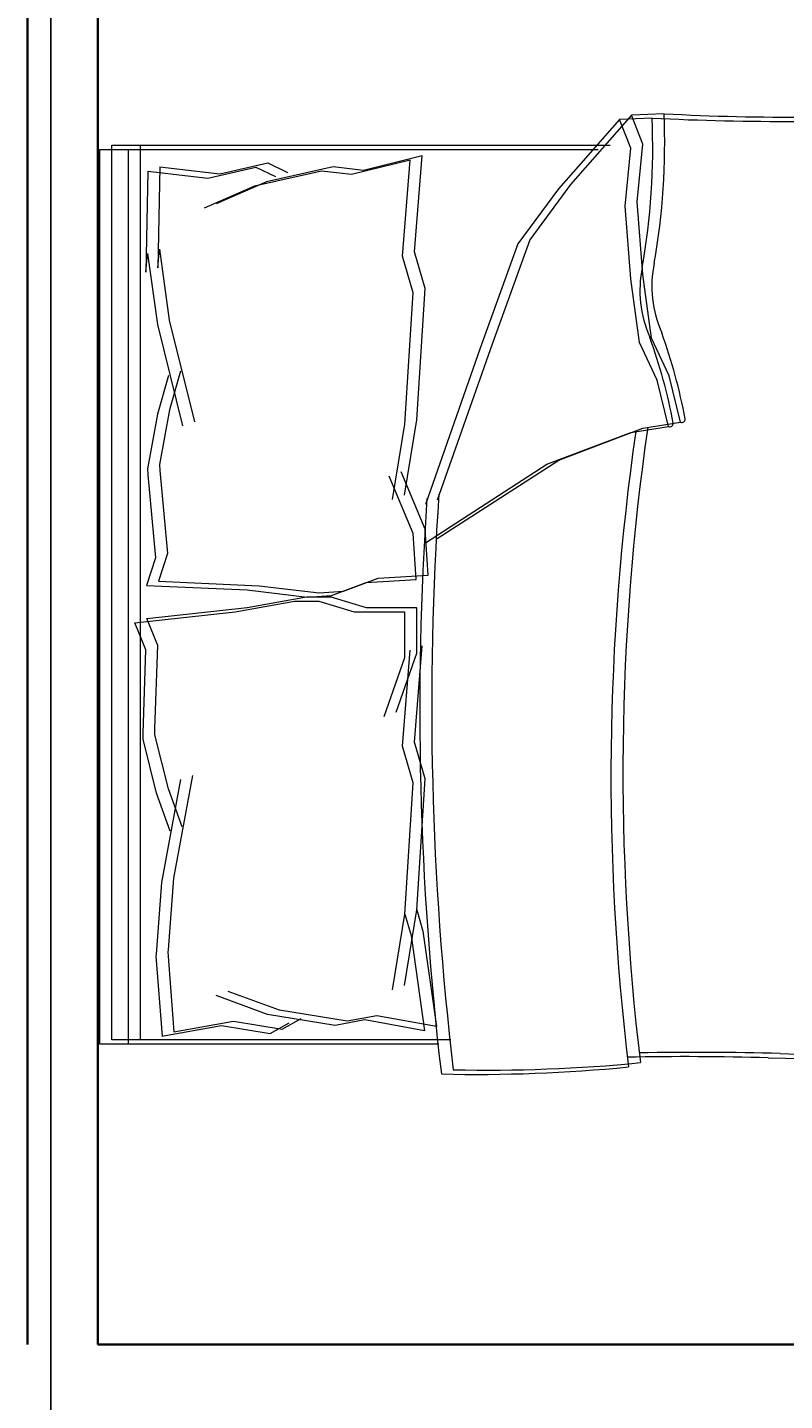
# Model space of a CAD drawing. Units: inches. Extents: x 1088 to 1703, y 668 to 1875.
# Tile 24 of 45: x 1436 to 1484, y 1416 to 1504. Entities that reach past the tile are written whole.
import ezdxf

# ---------------------------------------------------------------- set-up
doc = ezdxf.new("R2010")
doc.units = ezdxf.units.IN
for name, color, linetype, lineweight in [('A-ANNO-DIMS', 2, 'Continuous', 18), ('A-FURN', 8, 'Continuous', 13), ('A-WALL', 7, 'Continuous', 35)]:
    doc.layers.add(name, color=color, linetype=linetype, lineweight=lineweight)
doc.styles.get("Standard").update_dxf_attribs({"font": 'arial.ttf'})
doc.dimstyles.get("Standard").update_dxf_attribs({"dimtxt": 0.18, "dimasz": 0.18, "dimexe": 0.18, "dimexo": 0.0625, "dimgap": 0.09, "dimtad": 0, "dimtih": 1, "dimtoh": 1, "dimdec": 4, "dimzin": 0, "dimdsep": 46, "dimtxsty": 'Standard', "dimcen": 0.09, "dimadec": 0, "dimazin": 0, "dimtfac": 1, "dimtdec": 4, "dimtofl": 0, "dimtmove": 0, "dimatfit": 3, "dimfxl": 1, "dimtolj": 1, "dimtzin": 0, "dimarcsym": 0})

# ---------------------------------------------------------------- blocks, each defined once
blk = doc.blocks.new('BED-DOUBLE')
for p, q in [((33.263, 63.381), (29.367, 58.939)), ((34.03, 63.655), (30.133, 59.213)), ((35.355, 63.476), (33.263, 63.381, 4.641)), ((34.006, 61.538), (33.263, 63.381)), ((36.121, 63.75), (34.03, 63.655, 4.641)), ((34.772, 61.812), (34.03, 63.655)), ((0.766, 61.734), (32.668, 61.734)), ((0.766, 4.44), (0.766, 61.734)), ((2.605, 4.44), (2.605, 61.734)), ((34.401, 58.099), (34.772, 61.812)), ((0, 61.46), (31.901, 61.46)), ((0, 4.167), (0, 61.46)), ((1.838, 4.167), (1.838, 61.46)), ((19.868, 60.78), (16.105, 59.851)), ((20.635, 61.054), (16.872, 60.124)), ((19.384, 54.628), (19.868, 60.78)), ((20.151, 54.902), (20.635, 61.054)), ((33.634, 57.825), (34.006, 61.538)), ((3.065, 60.077), (2.949, 53.601)), ((3.065, 60.077), (6.915, 59.624)), ((3.832, 60.351), (3.716, 53.875)), ((3.832, 60.351), (7.681, 59.897)), ((6.915, 59.624), (9.996, 60.337)), ((7.681, 59.897), (10.763, 60.611)), ((14.181, 60.078), (9.899, 59.115)), ((9.996, 60.337), (11.251, 59.721)), ((14.947, 60.351), (10.665, 59.389)), ((10.763, 60.611), (12.017, 59.995)), ((16.105, 59.851), (14.181, 60.078)), ((16.872, 60.124), (14.947, 60.351)), ((9.899, 59.115), (6.688, 57.699)), ((10.665, 59.389), (7.454, 57.973)), ((29.367, 58.939), (26.769, 55.411)), ((30.133, 59.213), (27.535, 55.685)), ((34.772, 53.457), (34.401, 58.099)), ((34.006, 53.183), (33.634, 57.825)), ((26.769, 55.411), (24.357, 48.727)), ((27.535, 55.685), (25.123, 49.001)), ((2.949, 53.601), (3.048, 54.803)), ((3.048, 54.803), (3.68, 50.25)), ((3.716, 53.875), (3.814, 55.077)), ((3.814, 55.077), (4.446, 50.523)), ((20.052, 52.278), (19.384, 54.628)), ((20.819, 52.552), (20.151, 54.902)), ((34.562, 49.098), (34.006, 53.183)), ((35.329, 49.372), (34.772, 53.457)), ((19.536, 43.874), (20.052, 52.278)), ((20.302, 44.148), (20.819, 52.552)), ((3.68, 50.25), (5.301, 43.753)), ((4.446, 50.523), (6.068, 44.027)), ((36.442, 46.958), (35.329, 49.372)), ((24.357, 48.727), (20.84, 38.731)), ((25.123, 49.001), (21.606, 39.005)), ((35.676, 46.685), (34.562, 49.098)), ((4.404, 46.996), (3.69, 44.52)), ((5.171, 47.27), (4.457, 44.794)), ((36.418, 43.714), (35.676, 46.685)), ((37.184, 43.988), (36.442, 46.958)), ((3.69, 44.52), (3.042, 41.007)), ((4.457, 44.794), (3.808, 41.281)), ((19.503, 39.314), (20.302, 44.148)), ((34.772, 43.616), (37.184, 43.988)), ((18.736, 39.04), (19.536, 43.874)), ((28.624, 41.3), (34.006, 43.342)), ((29.391, 41.574), (34.772, 43.616)), ((34.006, 43.342), (36.418, 43.714)), ((21.606, 36.551), (29.391, 41.574)), ((3.042, 41.007), (3.066, 40.622)), ((3.066, 40.622), (3.571, 35.314)), ((3.808, 41.281), (3.832, 40.896)), ((3.832, 40.896), (4.338, 35.587)), ((20.068, 36.866), (18.528, 40.547)), ((20.835, 37.139), (19.294, 40.82)), ((20.84, 36.277), (28.624, 41.3)), ((21.018, 34.199), (20.835, 37.139)), ((20.252, 33.925), (20.068, 36.866)), ((3.571, 35.314), (2.987, 33.541)), ((4.338, 35.587), (3.754, 33.814)), ((2.987, 33.541), (9.432, 33.249)), ((3.754, 33.814), (10.198, 33.523)), ((10.198, 33.523), (14.047, 33.069)), ((14.838, 32.892), (17.044, 33.725)), ((15.604, 33.166), (17.81, 33.998)), ((17.044, 33.725), (20.252, 33.925)), ((17.81, 33.998), (21.018, 34.199)), ((9.422, 32.117), (13.236, 32.81)), ((9.432, 33.249), (13.281, 32.795)), ((13.236, 32.81), (14.796, 32.81)), ((13.281, 32.795), (14.838, 32.892)), ((14.047, 33.069), (15.604, 33.166)), ((14.796, 32.81), (17.049, 32.117)), ((2.242, 31.15), (8.656, 31.843)), ((3.008, 31.424), (9.422, 32.117)), ((8.656, 31.843), (12.469, 32.536)), ((12.469, 32.536), (14.029, 32.536)), ((14.029, 32.536), (16.283, 31.843)), ((16.283, 31.843), (19.497, 31.843)), ((17.049, 32.117), (20.264, 32.117)), ((19.497, 31.843), (19.497, 28.897)), ((20.264, 32.117), (20.264, 29.171)), ((2.935, 29.417), (2.242, 31.15)), ((3.702, 29.691), (3.008, 31.424)), ((2.762, 24.087), (2.935, 29.417)), ((3.528, 24.361), (3.702, 29.691)), ((20.264, 29.171), (18.956, 25.401)), ((19.384, 23.239), (19.868, 29.391)), ((20.151, 23.513), (20.635, 29.665)), ((19.497, 28.897), (18.189, 25.127)), ((2.762, 23.701), (2.762, 24.087)), ((3.528, 23.975), (3.528, 24.361)), ((4.395, 20.509), (3.528, 23.975)), ((3.629, 20.235), (2.762, 23.701)), ((20.052, 20.889), (19.384, 23.239)), ((20.819, 21.163), (20.151, 23.513)), ((4.742, 14.79), (5.955, 21.376)), ((20.302, 12.759), (20.819, 21.163)), ((4.495, 17.809), (3.629, 20.235)), ((3.975, 14.516), (5.189, 21.102)), ((5.262, 18.083), (4.395, 20.509)), ((19.536, 12.485), (20.052, 20.889)), ((3.629, 9.933), (3.975, 14.516)), ((4.395, 10.206), (4.742, 14.79)), ((18.736, 7.651), (19.536, 12.485)), ((19.503, 7.925), (20.302, 12.759)), ((19.536, 12.485), (19.923, 11.126)), ((20.302, 12.759), (20.689, 11.4)), ((19.923, 11.126), (20.789, 5.016)), ((20.689, 11.4), (21.556, 5.29)), ((3.607, 9.806), (3.629, 9.933)), ((4.002, 4.674), (3.607, 9.806)), ((4.373, 10.08), (4.395, 10.206)), ((4.768, 4.948), (4.373, 10.08)), ((10.736, 6.056), (7.442, 7.269)), ((11.502, 6.33), (8.209, 7.543)), ((15.836, 5.637), (11.502, 6.33)), ((3.975, 4.67), (7.789, 5.363)), ((4.742, 4.943), (8.555, 5.637)), ((7.789, 5.363), (10.909, 4.843)), ((8.555, 5.637), (11.675, 5.117)), ((15.069, 5.363), (10.736, 6.056)), ((10.909, 4.843), (12.122, 5.536)), ((11.675, 5.117), (12.889, 5.81)), ((16.976, 5.709), (15.069, 5.363)), ((17.742, 5.983), (15.836, 5.637)), ((20.789, 5.016), (16.976, 5.709)), ((21.556, 5.29), (17.742, 5.983)), ((22.478, 4.44), (0.766, 4.44)), ((21.712, 4.167), (0, 4.167))]:
    blk.add_line(p, q)
for centre, radius, start, end in [((-7.98, 61.534), 43.378, 349.87628, 2.56571), ((43.537, 218.511), 155.251, 266.97912, 273.83645), ((-7.213, 61.808), 43.378, 349.87628, 2.56571), ((44.303, 218.785), 155.251, 266.97912, 273.83645), ((42.039, 52.443), 7.462, 168.6608, 203.73842), ((42.806, 52.716), 7.462, 168.6608, 203.73842), ((1.777, 37.349), 35.551, 10.66171, 19.88058), ((2.543, 37.623), 35.551, 10.66171, 19.88058), ((37.259, 44.196), 0.221, 250.24637, 1.13765), ((187.401, 21.287), 154.676, 171.78449, 186.90062), ((188.167, 21.561), 154.676, 171.78449, 186.90062), ((36.492, 43.922), 0.221, 250.24637, 1.13765), ((218.255, 25.607), 197.774, 176.08655, 186.78213), ((219.021, 25.88), 197.774, 176.08655, 186.78213), ((38.139, -200.304), 203.938, 88.4762, 91.00819), ((61.445, 581.507), 578.221, 268.227709, 271.718541), ((24.093, 102.097), 99.872, 268.72178, 275.60397), ((24.859, 102.371), 99.872, 268.72178, 275.60397), ((37.373, -200.577), 203.938, 88.4762, 91.00819), ((60.679, 581.233), 578.221, 268.227709, 271.718541)]:
    blk.add_arc(centre, radius, start, end)
blk = doc.blocks.new('*D38')
at = {"layer": 'A-ANNO-DIMS', "color": 0, "lineweight": -2, "transparency": 16777216}
for p, q in [((1317.345, 1736.945), (1317.345, 725.549)), ((1437.345, 1736.945), (1437.345, 725.549)), ((1317.525, 725.729), (1377.065, 725.729)), ((1437.165, 725.729), (1377.625, 725.729))]:
    blk.add_line(p, q, dxfattribs=at)
at = {"layer": 'A-ANNO-DIMS', "color": 0, "transparency": 16777216}
for points in [[(1317.525, 725.759), (1317.525, 725.699), (1317.345, 725.729)], [(1437.165, 725.759), (1437.165, 725.699), (1437.345, 725.729)]]:
    blk.add_solid(points, dxfattribs=at)
at = {"layer": 'Defpoints', "color": 0, "transparency": 16777216}
for p in [(1317.345, 1737.007), (1437.345, 1737.007), (1437.345, 725.729)]:
    blk.add_point(p, dxfattribs=at)
at = {"layer": 'A-ANNO-DIMS', "color": 0, "transparency": 16777216, "insert": (1377.345, 725.729), "char_height": 0.18, "attachment_point": 5}
blk.add_mtext('\\A1;120', dxfattribs=at)

msp = doc.modelspace()

# ---------------------------------------------------------------- linework, layer by layer
at = {"layer": 'A-WALL'}
for p, q in [((1435.845, 1419.558), (1435.845, 1539.558)), ((1440.345, 1419.558), (1440.345, 1539.583)), ((1435.845, 1419.558), (1435.845, 1445.058)), ((1585.845, 1419.558), (1440.345, 1419.558))]:
    msp.add_line(p, q, dxfattribs=at)

# ---------------------------------------------------------------- block references
at = {"layer": 'A-FURN'}
msp.add_blockref('BED-DOUBLE', (1440.48, 1434.64), dxfattribs=at)

# ---------------------------------------------------------------- dimensions: what is measured, and where the dimension line sits
at = {"layer": 'A-ANNO-DIMS'}
dim = msp.add_linear_dim(base=(1437.345, 725.729), p1=(1317.345, 1737.007), p2=(1437.345, 1737.007), dimstyle='Standard', override={"dimdec": 0, "dimlfac": 1, "dimrnd": 0, "dimzin": 0, "dimdsep": 46, "dimlunit": 2}, dxfattribs=at)
dim.commit()
dim.dimension.update_dxf_attribs({"geometry": '*D38', "text_midpoint": (1377.345, 725.729)})

doc.saveas('drawing.dxf')
